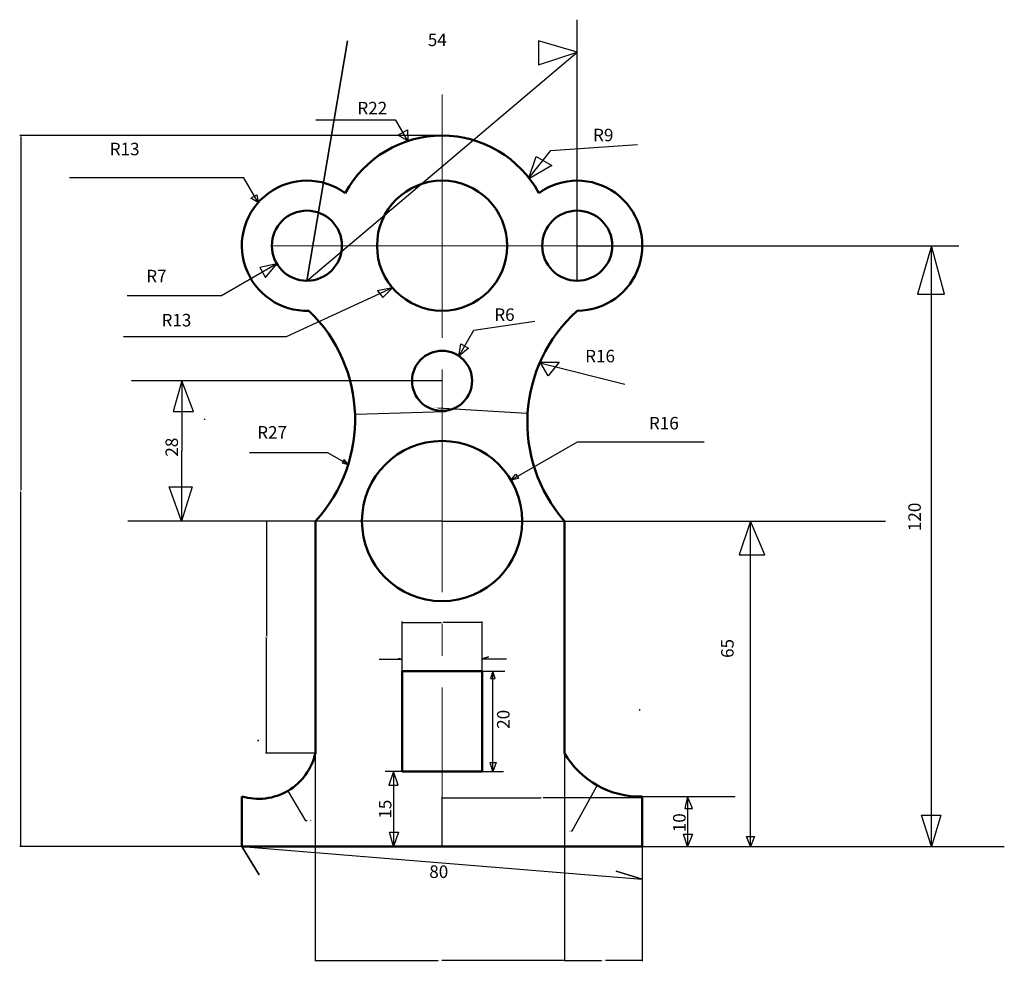
# Model space of a CAD drawing. Units: inches. Extents: x 132205 to 264922, y 44864 to 89774.
# Tile 1 of 1: x 132205.3 to 132402, y 44864.1 to 45052.2. Entities that reach past the tile are written whole.
import ezdxf

# ---------------------------------------------------------------- set-up
doc = ezdxf.new("R2010")
doc.units = ezdxf.units.IN
doc.linetypes.add('CENTER', pattern=[50.8, 31.75, -6.35, 6.35, -6.35])
for name, color, linetype, lineweight in [('M-CNTR', 4, 'CENTER', 18), ('M-DIMS', 2, 'Continuous', 25), ('M-OUTL', 7, 'Continuous', 50), ('M-TEXT', 7, 'Continuous', 25)]:
    doc.layers.add(name, color=color, linetype=linetype, lineweight=lineweight)
doc.styles.get("Standard").update_dxf_attribs({"font": 'arial.ttf'})
doc.dimstyles.get("Standard").update_dxf_attribs({"dimtxt": 0.18, "dimasz": 0.18, "dimexe": 0.18, "dimexo": 0.0625, "dimgap": 0.09, "dimtad": 0, "dimtih": 1, "dimtoh": 1, "dimdec": 4, "dimzin": 0, "dimdsep": 46, "dimtxsty": 'Standard', "dimcen": 0.09, "dimadec": 0, "dimazin": 0, "dimtfac": 1, "dimtdec": 4, "dimtofl": 0, "dimtmove": 0, "dimatfit": 3, "dimfxl": 1, "dimtolj": 1, "dimtzin": 0, "dimarcsym": 0})

# ---------------------------------------------------------------- blocks, each defined once
blk = doc.blocks.new('HOLE-D14')
blk.add_circle((7, 7), 7)
blk = doc.blocks.new('*D2')
at = {"layer": 'Defpoints', "color": 0, "transparency": 16777216}
for p in [(132205.48, 45029.04), (132289.66, 45029.04), (132249.66, 44887.04)]:
    blk.add_point(p, dxfattribs=at)
at = {"layer": 'M-DIMS', "color": 0, "lineweight": -2, "transparency": 16777216}
for p, q in [((132289.6, 45029.04), (132205.3, 45029.04)), ((132205.48, 45028.86), (132205.48, 44958.22)), ((132205.48, 44887.22), (132205.48, 44957.86)), ((132249.6, 44887.04), (132205.3, 44887.04))]:
    blk.add_line(p, q, dxfattribs=at)
at = {"layer": 'M-DIMS', "color": 0, "transparency": 16777216}
for points in [[(132205.45, 45028.86), (132205.51, 45028.86), (132205.48, 45029.04)], [(132205.45, 44887.22), (132205.51, 44887.22), (132205.48, 44887.04)]]:
    blk.add_solid(points, dxfattribs=at)
at = {"layer": 'M-DIMS', "color": 0, "transparency": 16777216, "insert": (132205.48, 44958.04), "char_height": 0.18, "attachment_point": 5}
blk.add_mtext('\\A1;142', dxfattribs=at)
blk = doc.blocks.new('*D3')
at = {"layer": 'Defpoints', "color": 0, "transparency": 16777216}
for p in [(132297.66, 44931.79), (132281.66, 44922.04), (132297.66, 44922.04)]:
    blk.add_point(p, dxfattribs=at)
at = {"layer": 'M-DIMS', "color": 0, "lineweight": -2, "transparency": 16777216}
for p, q in [((132281.66, 44922.1), (132281.66, 44931.97)), ((132281.84, 44931.79), (132289.45, 44931.79)), ((132297.48, 44931.79), (132289.87, 44931.79)), ((132297.66, 44922.1), (132297.66, 44931.97))]:
    blk.add_line(p, q, dxfattribs=at)
at = {"layer": 'M-DIMS', "color": 0, "transparency": 16777216}
for points in [[(132281.84, 44931.82), (132281.84, 44931.76), (132281.66, 44931.79)], [(132297.48, 44931.82), (132297.48, 44931.76), (132297.66, 44931.79)]]:
    blk.add_solid(points, dxfattribs=at)
at = {"layer": 'M-DIMS', "color": 0, "transparency": 16777216, "insert": (132289.66, 44931.79), "char_height": 0.18, "attachment_point": 5}
blk.add_mtext('\\A1;16', dxfattribs=at)
blk = doc.blocks.new('*D4')
at = {"layer": 'Defpoints', "color": 0, "transparency": 16777216}
for p in [(132264.34, 44905.71), (132314.12, 44905.71), (132314.12, 44864.29)]:
    blk.add_point(p, dxfattribs=at)
at = {"layer": 'M-DIMS', "color": 0, "lineweight": -2, "transparency": 16777216}
for p, q in [((132264.34, 44905.65), (132264.34, 44864.11)), ((132314.12, 44905.65), (132314.12, 44864.11)), ((132264.52, 44864.29), (132288.84, 44864.29)), ((132313.94, 44864.29), (132289.63, 44864.29))]:
    blk.add_line(p, q, dxfattribs=at)
at = {"layer": 'M-DIMS', "color": 0, "transparency": 16777216}
for points in [[(132264.52, 44864.32), (132264.52, 44864.26), (132264.34, 44864.29)], [(132313.94, 44864.32), (132313.94, 44864.26), (132314.12, 44864.29)]]:
    blk.add_solid(points, dxfattribs=at)
at = {"layer": 'M-DIMS', "color": 0, "transparency": 16777216, "insert": (132289.23, 44864.29), "char_height": 0.18, "attachment_point": 5}
blk.add_mtext('\\A1;49.78', dxfattribs=at)
blk = doc.blocks.new('*D5')
at = {"layer": 'Defpoints', "color": 0, "transparency": 16777216}
for p in [(132314.12, 44905.71), (132329.66, 44897.04), (132329.66, 44864.29)]:
    blk.add_point(p, dxfattribs=at)
at = {"layer": 'M-DIMS', "color": 0, "lineweight": -2, "transparency": 16777216}
for p, q in [((132314.12, 44905.65), (132314.12, 44864.11)), ((132329.66, 44896.97), (132329.66, 44864.11)), ((132314.3, 44864.29), (132321.51, 44864.29)), ((132329.48, 44864.29), (132322.28, 44864.29))]:
    blk.add_line(p, q, dxfattribs=at)
at = {"layer": 'M-DIMS', "color": 0, "transparency": 16777216}
for points in [[(132314.3, 44864.32), (132314.3, 44864.26), (132314.12, 44864.29)], [(132329.48, 44864.32), (132329.48, 44864.26), (132329.66, 44864.29)]]:
    blk.add_solid(points, dxfattribs=at)
at = {"layer": 'M-DIMS', "color": 0, "transparency": 16777216, "insert": (132321.89, 44864.29), "char_height": 0.18, "attachment_point": 5}
blk.add_mtext('\\A1;15.54', dxfattribs=at)
blk = doc.blocks.new('*D6')
at = {"layer": 'Defpoints', "color": 0, "transparency": 16777216}
for p in [(132254.59, 44952.04), (132264.34, 44952.04), (132264.34, 44905.71)]:
    blk.add_point(p, dxfattribs=at)
at = {"layer": 'M-DIMS', "color": 0, "lineweight": -2, "transparency": 16777216}
for p, q in [((132264.28, 44952.04), (132254.41, 44952.04)), ((132254.59, 44951.86), (132254.59, 44929.06)), ((132254.59, 44905.89), (132254.59, 44928.69)), ((132264.28, 44905.71), (132254.41, 44905.71))]:
    blk.add_line(p, q, dxfattribs=at)
at = {"layer": 'M-DIMS', "color": 0, "transparency": 16777216}
for points in [[(132254.56, 44951.86), (132254.62, 44951.86), (132254.59, 44952.04)], [(132254.56, 44905.89), (132254.62, 44905.89), (132254.59, 44905.71)]]:
    blk.add_solid(points, dxfattribs=at)
at = {"layer": 'M-DIMS', "color": 0, "transparency": 16777216, "insert": (132254.59, 44928.87), "char_height": 0.18, "attachment_point": 5}
blk.add_mtext('\\A1;46.33', dxfattribs=at)
blk = doc.blocks.new('*D7')
at = {"layer": 'Defpoints', "color": 0, "transparency": 16777216}
for p in [(132329.66, 44896.79), (132289.66, 44887.04), (132329.66, 44887.04)]:
    blk.add_point(p, dxfattribs=at)
at = {"layer": 'M-DIMS', "color": 0, "lineweight": -2, "transparency": 16777216}
for p, q in [((132289.66, 44887.1), (132289.66, 44896.97)), ((132289.84, 44896.79), (132309.44, 44896.79)), ((132329.48, 44896.79), (132309.88, 44896.79)), ((132329.66, 44887.1), (132329.66, 44896.97))]:
    blk.add_line(p, q, dxfattribs=at)
at = {"layer": 'M-DIMS', "color": 0, "transparency": 16777216}
for points in [[(132289.84, 44896.82), (132289.84, 44896.76), (132289.66, 44896.79)], [(132329.48, 44896.82), (132329.48, 44896.76), (132329.66, 44896.79)]]:
    blk.add_solid(points, dxfattribs=at)
at = {"layer": 'M-DIMS', "color": 0, "transparency": 16777216, "insert": (132309.66, 44896.79), "char_height": 0.18, "attachment_point": 5}
blk.add_mtext('\\A1;40', dxfattribs=at)
blk = doc.blocks.new('*D8')
at = {"layer": 'Defpoints', "color": 0, "transparency": 16777216}
for p in [(132329.14, 44914.37), (132320.69, 44899.23)]:
    blk.add_point(p, dxfattribs=at)
at = {"layer": 'M-DIMS', "color": 0, "lineweight": -2, "transparency": 16777216}
for p, q in [((132329.05, 44914.37), (132329.23, 44914.37)), ((132329.14, 44914.28), (132329.14, 44914.46)), ((132315.62, 44890.14), (132320.61, 44899.07)), ((132315.44, 44890.14), (132315.62, 44890.14))]:
    blk.add_line(p, q, dxfattribs=at)
at = {"layer": 'M-DIMS', "color": 0, "transparency": 16777216}
blk.add_solid([(132320.58, 44899.09), (132320.63, 44899.06), (132320.69, 44899.23)], dxfattribs=at)
at = {"layer": 'M-DIMS', "color": 0, "transparency": 16777216, "insert": (132314.89, 44890.14), "char_height": 0.18, "attachment_point": 5}
blk.add_mtext('\\A1;R17.343', dxfattribs=at)
blk = doc.blocks.new('*D9')
at = {"layer": 'Defpoints', "color": 0, "transparency": 16777216}
for p in [(132252.95, 44908.24), (132258.88, 44898.19)]:
    blk.add_point(p, dxfattribs=at)
at = {"layer": 'M-DIMS', "color": 0, "lineweight": -2, "transparency": 16777216}
for p, q in [((132252.86, 44908.24), (132253.04, 44908.24)), ((132252.95, 44908.15), (132252.95, 44908.33)), ((132262.45, 44892.16), (132258.98, 44898.03)), ((132262.63, 44892.16), (132262.45, 44892.16))]:
    blk.add_line(p, q, dxfattribs=at)
at = {"layer": 'M-DIMS', "color": 0, "transparency": 16777216}
blk.add_solid([(132259, 44898.05), (132258.95, 44898.02), (132258.88, 44898.19)], dxfattribs=at)
at = {"layer": 'M-DIMS', "color": 0, "transparency": 16777216, "insert": (132263.18, 44892.16), "char_height": 0.18, "attachment_point": 5}
blk.add_mtext('\\A1;R11.673', dxfattribs=at)
blk = doc.blocks.new('*D10')
at = {"layer": 'Defpoints', "color": 0, "transparency": 16777216}
for p in [(132242.26, 44972.38), (132272.28, 44973.3)]:
    blk.add_point(p, dxfattribs=at)
at = {"layer": 'M-DIMS', "color": 0, "lineweight": -2, "transparency": 16777216}
for p, q in [((132242.17, 44972.38), (132242.35, 44972.38)), ((132242.26, 44972.29), (132242.26, 44972.47)), ((132290.28, 44973.85), (132272.46, 44973.31))]:
    blk.add_line(p, q, dxfattribs=at)
at = {"layer": 'M-DIMS', "color": 0, "transparency": 16777216}
blk.add_solid([(132272.45, 44973.34), (132272.46, 44973.28), (132272.28, 44973.3)], dxfattribs=at)
at = {"layer": 'M-DIMS', "color": 0, "transparency": 16777216, "insert": (132290.83, 44973.85), "char_height": 0.18, "attachment_point": 5}
blk.add_mtext('\\A1;R30.027', dxfattribs=at)
blk = doc.blocks.new('*D11')
at = {"layer": 'Defpoints', "color": 0, "transparency": 16777216}
for p in [(132306.76, 44973.56), (132336.61, 44971.75)]:
    blk.add_point(p, dxfattribs=at)
at = {"layer": 'M-DIMS', "color": 0, "lineweight": -2, "transparency": 16777216}
for p, q in [((132288.84, 44974.64), (132306.58, 44973.57)), ((132336.52, 44971.75), (132336.7, 44971.75)), ((132336.61, 44971.66), (132336.61, 44971.84))]:
    blk.add_line(p, q, dxfattribs=at)
at = {"layer": 'M-DIMS', "color": 0, "transparency": 16777216}
blk.add_solid([(132306.58, 44973.6), (132306.58, 44973.54), (132306.76, 44973.56)], dxfattribs=at)
at = {"layer": 'M-DIMS', "color": 0, "transparency": 16777216, "insert": (132288.38, 44974.64), "char_height": 0.18, "attachment_point": 5}
blk.add_mtext('\\A1;R29.91', dxfattribs=at)

msp = doc.modelspace()

# ---------------------------------------------------------------- linework, layer by layer
at = {"layer": 'M-CNTR'}
for p, q in [((132289.6611, 45007.0374), (132289.6611, 45037.202)), ((132267.6611, 45007.0374), (132255.6611, 45007.0374)), ((132289.6611, 45007.0374), (132267.6611, 45007.0374)), ((132289.6611, 44887.0374), (132289.6611, 45007.0374)), ((132289.6611, 45007.0374), (132316.6611, 45007.0374)), ((132289.6611, 44952.0374), (132289.6611, 44980.0374)), ((132289.6611, 44887.0374), (132289.6611, 44952.0374)), ((132289.6611, 44887.0374), (132289.6611, 44902.0374))]:
    msp.add_line(p, q, dxfattribs=at)
at = {"layer": 'M-DIMS'}
for p, q in [((132316.6611, 45000.0374), (132316.6611, 45052.1727)), ((132262.6611, 45000.0374, 1990.0236), (132270.7604, 45047.9723)), ((132270.7604, 45047.9723, -203.1204), (132262.6611, 45000.0374, 1990.0236)), ((132270.7604, 45047.9723), (132270.7604, 45047.9723, -203.1204)), ((132316.6611, 45045.6911), (132308.9178, 45047.92)), ((132308.9178, 45047.92), (132308.9178, 45043.152)), ((132262.6611, 45000.0374, 1990.0236), (132316.6611, 45045.6911)), ((132308.9178, 45043.152), (132316.6538, 45045.685, 0.268)), ((132280.4359, 45032.1182), (132264.446, 45032.1182)), ((132282.8404, 45027.9534), (132280.4359, 45032.1182)), ((132280.8504, 45029.1023), (132282.7383, 45030.1922)), ((132282.7383, 45030.1922), (132282.8404, 45027.9534)), ((132282.8404, 45027.9534), (132280.8504, 45029.1023)), ((132307.0224, 45020.5498), (132311.4005, 45026.0764)), ((132311.4005, 45026.0764), (132328.7053, 45027.2352)), ((132307.0224, 45020.5498), (132308.4409, 45024.8487)), ((132308.4409, 45024.8487), (132311.6031, 45023.0231)), ((132311.6031, 45023.0231), (132307.114, 45020.4313)), ((132250.0716, 45020.5823), (132215.2334, 45020.5823)), ((132252.9209, 45015.6472), (132250.0716, 45020.5823)), ((132251.4384, 45016.5031), (132252.628, 45017.1899)), ((132252.9209, 45015.6472), (132251.4384, 45016.5031)), ((132252.628, 45017.1899), (132252.9209, 45015.6472)), ((132252.9209, 45015.6472), (132252.9209, 45015.6472)), ((132316.6611, 45007.0374), (132392.9299, 45007.0374)), ((132387.4093, 45007.0374), (132384.6349, 44997.3858)), ((132387.4093, 44887.0374), (132387.4093, 45007.0374)), ((132390.0528, 44997.3858), (132387.4093, 45007.0374)), ((132256.6723, 45003.4133), (132245.6104, 44997.0266)), ((132256.6723, 45003.4133), (132253.2638, 45002.6493)), ((132253.2638, 45002.6493), (132254.3948, 45000.6904)), ((132254.3948, 45000.6904), (132256.6723, 45003.4133)), ((132262.6611, 45000.0374), (132262.6611, 45000.0374, 2281.6152)), ((132279.7741, 44998.5966), (132258.541, 44988.8291)), ((132279.7741, 44998.5966), (132276.7557, 44998.0513)), ((132276.7557, 44998.0513), (132277.8375, 44996.706)), ((132277.8375, 44996.706), (132279.7741, 44998.5966)), ((132245.6104, 44997.0266), (132226.7761, 44997.0266)), ((132384.6349, 44997.3858), (132390.0528, 44997.3858)), ((132293.036, 44984.9983), (132296.015, 44990.158)), ((132296.015, 44990.158), (132308.1721, 44991.9752)), ((132258.541, 44988.8291), (132226.01, 44988.8291)), ((132293.036, 44984.9983), (132293.4136, 44987.4392)), ((132294.9687, 44986.5415), (132293.036, 44984.9983)), ((132293.4136, 44987.4392), (132294.9687, 44986.5415)), ((132309.1747, 44983.6612), (132326.1454, 44979.3804)), ((132310.8241, 44981.0609), (132309.2385, 44983.8072)), ((132309.2385, 44983.8072), (132313.0577, 44983.8072)), ((132313.0577, 44983.8072), (132310.8241, 44981.0609)), ((132289.6611, 44980.0374), (132227.5826, 44980.0374)), ((132237.6433, 44980.0374), (132235.9475, 44973.9)), ((132237.6433, 44980.0374), (132237.6049, 44952.0374)), ((132240.0064, 44973.9), (132237.6433, 44980.0374)), ((132235.9475, 44973.9), (132240.0064, 44973.9)), ((132303.4116, 44960.2181), (132316.7081, 44967.8948)), ((132316.7081, 44967.8948), (132342.0004, 44967.8948)), ((132266.8613, 44965.6984), (132251.2163, 44965.6984)), ((132270.903, 44963.3649), (132266.8613, 44965.6984)), ((132270.0968, 44964.3328), (132269.7046, 44963.6535)), ((132269.7046, 44963.6535), (132270.903, 44963.3649)), ((132270.903, 44963.3649), (132270.0968, 44964.3328)), ((132303.4116, 44960.2181), (132304.3976, 44961.4052)), ((132304.3976, 44961.4052), (132304.8998, 44960.5354)), ((132237.6049, 44952.0374), (132235.1148, 44958.8887)), ((132235.1148, 44958.8887), (132239.7161, 44958.8887)), ((132239.7161, 44958.8887), (132237.6049, 44952.0374)), ((132304.8998, 44960.5354), (132303.4116, 44960.2181)), ((132289.6611, 44952.0374), (132226.8674, 44952.0374)), ((132289.6611, 44952.0374), (132378.2196, 44952.0374)), ((132351.2485, 44952.0374), (132349.0123, 44945.2761)), ((132351.2485, 44887.0374), (132351.2485, 44952.0374)), ((132354.1555, 44945.2761), (132351.2485, 44952.0374)), ((132349.0123, 44945.2761), (132354.1555, 44945.2761)), ((132281.6611, 44922.0374), (132281.6611, 44926.6883)), ((132297.6611, 44922.0374), (132297.6611, 44927.0114)), ((132281.6611, 44924.3628), (132277.1216, 44924.3628)), ((132281.6611, 44924.3628), (132280.9291, 44924.6054)), ((132280.9291, 44924.6054), (132280.9291, 44924.6054, -20.4972)), ((132280.9291, 44924.6054, -20.4972), (132281.6611, 44924.3628)), ((132297.6611, 44924.5244), (132298.9141, 44924.9226)), ((132298.9141, 44924.9226, -32.5417), (132297.6611, 44924.5244)), ((132297.6611, 44924.5244), (132302.5499, 44924.5244)), ((132298.9141, 44924.9226), (132298.9141, 44924.9226, -32.5417)), ((132297.6611, 44922.0374), (132302.1854, 44922.0374)), ((132299.8005, 44922.0374), (132299.3286, 44920.5639)), ((132299.8005, 44902.0374), (132299.8005, 44922.0374)), ((132300.2787, 44920.5639), (132299.8005, 44922.0374)), ((132299.3286, 44920.5639), (132300.2787, 44920.5639)), ((132299.8005, 44902.0374), (132299.2642, 44903.8161)), ((132299.2642, 44903.8161), (132300.4403, 44903.8161)), ((132300.4403, 44903.8161), (132299.8005, 44902.0374)), ((132281.6611, 44902.0374), (132278.2953, 44902.0374)), ((132279.9782, 44902.0374), (132279.0417, 44899.2923)), ((132279.9782, 44902.0374), (132279.9782, 44887.0374)), ((132280.9046, 44899.2923), (132279.9782, 44902.0374)), ((132297.6611, 44902.0374), (132301.9399, 44902.0374)), ((132279.0417, 44899.2923), (132280.9046, 44899.2923)), ((132329.1443, 44897.0297), (132348.2397, 44897.0297)), ((132338.692, 44897.0297), (132338.1352, 44894.6311)), ((132338.692, 44897.0297), (132338.692, 44887.0374)), ((132339.7178, 44894.6311), (132338.692, 44897.0297)), ((132338.1352, 44894.6311), (132339.7178, 44894.6311)), ((132387.4093, 44887.0374), (132385.4378, 44893.3167)), ((132385.4378, 44893.3167), (132389.3021, 44893.3167)), ((132389.3021, 44893.3167), (132387.4093, 44887.0374)), ((132279.9782, 44887.0374), (132279.1464, 44889.8803)), ((132279.1464, 44889.8803), (132280.9467, 44889.8803)), ((132280.9467, 44889.8803), (132279.9782, 44887.0374)), ((132338.692, 44887.0374), (132337.8769, 44889.4848)), ((132337.8769, 44889.4848), (132339.6605, 44889.4848)), ((132339.6605, 44889.4848), (132338.692, 44887.0374)), ((132351.2485, 44887.0374), (132350.4727, 44889.0236)), ((132350.4727, 44889.0236), (132352.079, 44889.0236)), ((132352.079, 44889.0236), (132351.2485, 44887.0374)), ((132249.6611, 44887.0374), (132249.6611, 44887.0374, -577.5998)), ((132249.6611, 44887.0374, -288.7999), (132329.6611, 44880.5412)), ((132249.6611, 44887.0374, -288.7999), (132253.1439, 44881.3519)), ((132253.1439, 44881.3519, -86.8138), (132249.6611, 44887.0374, -288.7999)), ((132329.6611, 44887.0374), (132329.6611, 44874.0449)), ((132329.6611, 44887.0374), (132372.8359, 44887.0374)), ((132372.8359, 44887.0374), (132401.9827, 44887.0374)), ((132329.6611, 44880.5412), (132324.4569, 44882.1172)), ((132324.4569, 44882.1172), (132324.4569, 44882.1172, -147.5144)), ((132324.4569, 44882.1172, -147.5144), (132329.6611, 44880.5412)), ((132253.1439, 44881.3519), (132253.1439, 44881.3519, -86.8138))]:
    msp.add_line(p, q, dxfattribs=at)
at = {"layer": 'M-OUTL'}
for p, q in [((132264.3448, 44952.0374), (132264.3448, 44905.709)), ((132314.1202, 44952.0374), (132314.1202, 44905.709)), ((132297.6611, 44922.0374), (132281.6611, 44922.0374)), ((132281.6611, 44922.0374), (132281.6611, 44902.0374)), ((132297.6611, 44902.0374), (132297.6611, 44922.0374)), ((132281.6611, 44902.0374), (132289.6611, 44902.0374)), ((132289.6611, 44902.0374), (132297.6611, 44902.0374)), ((132249.6611, 44887.0374), (132249.6611, 44897.0374)), ((132329.6611, 44887.0374), (132329.6611, 44897.0374)), ((132249.6611, 44887.0374), (132329.6611, 44887.0374))]:
    msp.add_line(p, q, dxfattribs=at)
for centre, radius in [((132289.6611, 45007.0374), 13), ((132289.6611, 44980.0374), 6), ((132289.6611, 44952.0374), 16)]:
    msp.add_circle(centre, radius, dxfattribs=at)
for centre, radius, start, end in [((132289.6611, 45007.0374), 22, 28.50351, 151.49649), ((132262.6611, 45007.0374), 13, 53.861185, 271.75343), ((132316.6611, 45007.0374), 13, 270, 126.138815), ((132242.263, 44972.3842), 30.0266, 317.341721, 46.165139), ((132336.6128, 44971.7535), 29.9106, 131.839433, 221.236558), ((132252.9487, 44908.2383), 11.6734, 253.642398, 347.486417), ((132329.1443, 44914.3729), 17.3432, 209.970629, 271.707466)]:
    msp.add_arc(centre, radius, start, end, dxfattribs=at)

# ---------------------------------------------------------------- block references
for p in [(132255.661, 45000.037), (132309.661, 45000.037)]:
    msp.add_blockref('HOLE-D14', p, dxfattribs=at)

# ---------------------------------------------------------------- texts
at = {"layer": 'M-TEXT', "char_height": 2.5, "attachment_point": 1}
for s, width, insert in [('54', 8.275122, (132286.8115, 45049.4062)), ('R22', 4.479805, (132272.7465, 45035.7641)), ('R9', 3.937322, (132319.8304, 45030.3896)), ('R13', 11.824388, (132223.2755, 45027.5934)), ('R7', 7.028316, (132230.5672, 45002.2183)), ('R6', 4.524057, (132300.0957, 44994.5114)), ('R13', 8.402557, (132233.6211, 44993.416)), ('R16', 8.34049, (132318.2507, 44986.2333)), ('R16', 10.168, (132330.9875, 44972.8352)), ('R27', 5.65094, (132252.7292, 44971.0003)), ('80', 4.876442, (132287.1068, 44883.2611))]:
    msp.add_mtext_dynamic_manual_height_columns(s, width=width, gutter_width=12.5, heights=[0], dxfattribs=dict(at, insert=insert))
at = {"layer": 'M-TEXT', "char_height": 2.5, "attachment_point": 1, "rotation": 90}
for s, width, insert in [('28', 2.713767, (132234.404, 44964.9039)), ('120', 5.195146, (132382.807, 44950.0339)), ('65', 5.515361, (132345.409, 44924.7053)), ('20', 3.391643, (132300.6413, 44910.5529)), ('15', 1.881645, (132277.0448, 44892.6027)), ('10', 2.772137, (132335.8132, 44889.8937))]:
    msp.add_mtext_dynamic_manual_height_columns(s, width=width, gutter_width=12.5, heights=[0], dxfattribs=dict(at, insert=insert))

# ---------------------------------------------------------------- dimensions: what is measured, and where the dimension line sits
at = {"layer": 'M-DIMS'}
for base, p1, p2, override, picture, middle in [((132205.4834, 45029.0374), (132249.6611, 44887.0374), (132289.6611, 45029.0374), {"dimdec": 0, "dimlfac": 1, "dimrnd": 0, "dimzin": 0, "dimdsep": 46, "dimlunit": 2}, '*D2', (132205.4834, 44958.0374)), ((132254.5948, 44952.0374), (132264.3448, 44905.709), (132264.3448, 44952.0374), {"dimdec": 2, "dimlfac": 1, "dimrnd": 0, "dimzin": 0, "dimdsep": 46, "dimlunit": 2}, '*D6', (132254.5948, 44928.8732))]:
    dim = msp.add_linear_dim(base=base, p1=p1, p2=p2, angle=90, dimstyle='Standard', override=override, dxfattribs=at)
    dim.commit()
    dim.dimension.update_dxf_attribs({"geometry": picture, "text_midpoint": middle})
for center, mpoint, override, picture, middle in [((132336.6128, 44971.7535), (132306.7569, 44973.56), {"dimdec": 2, "dimlfac": 1, "dimrnd": 0, "dimzin": 0, "dimdsep": 46, "dimlunit": 2}, '*D11', (132288.8433, 44974.6439)), ((132242.263, 44972.3842), (132272.2755, 44973.303), {"dimdec": 3, "dimlfac": 1, "dimrnd": 0, "dimzin": 0, "dimdsep": 46, "dimlunit": 2}, '*D10', (132290.2831, 44973.8543)), ((132329.1443, 44914.3729), (132320.6939, 44899.2278), {"dimdec": 3, "dimlfac": 1, "dimrnd": 0, "dimzin": 0, "dimdsep": 46, "dimlunit": 2}, '*D8', (132314.8938, 44890.1407)), ((132252.9487, 44908.2383), (132258.885, 44898.187), {"dimdec": 3, "dimlfac": 1, "dimrnd": 0, "dimzin": 0, "dimdsep": 46, "dimlunit": 2}, '*D9', (132263.1765, 44892.1562))]:
    dim = msp.add_radius_dim(center=center, mpoint=mpoint, dimstyle='Standard', override=override, dxfattribs=at)
    dim.commit()
    dim.dimension.update_dxf_attribs({"geometry": picture, "text_midpoint": middle, "dimtype": 164})
for base, p1, p2, override, picture, middle in [((132297.6611, 44931.7874), (132281.6611, 44922.0374), (132297.6611, 44922.0374), {"dimdec": 0, "dimlfac": 1, "dimrnd": 0, "dimzin": 0, "dimdsep": 46, "dimlunit": 2}, '*D3', (132289.6611, 44931.7874)), ((132314.1202, 44864.2949), (132264.3448, 44905.709), (132314.1202, 44905.709), {"dimdec": 2, "dimlfac": 1, "dimrnd": 0, "dimzin": 0, "dimdsep": 46, "dimlunit": 2}, '*D4', (132289.2325, 44864.2949)), ((132329.6611, 44864.2949), (132314.1202, 44905.709), (132329.6611, 44897.0374), {"dimdec": 2, "dimlfac": 1, "dimrnd": 0, "dimzin": 0, "dimdsep": 46, "dimlunit": 2}, '*D5', (132321.8907, 44864.2949)), ((132329.6611, 44896.7874), (132289.6611, 44887.0374), (132329.6611, 44887.0374), {"dimdec": 0, "dimlfac": 1, "dimrnd": 0, "dimzin": 0, "dimdsep": 46, "dimlunit": 2}, '*D7', (132309.6611, 44896.7874))]:
    dim = msp.add_linear_dim(base=base, p1=p1, p2=p2, dimstyle='Standard', override=override, dxfattribs=at)
    dim.commit()
    dim.dimension.update_dxf_attribs({"geometry": picture, "text_midpoint": middle})

doc.saveas('drawing.dxf')
